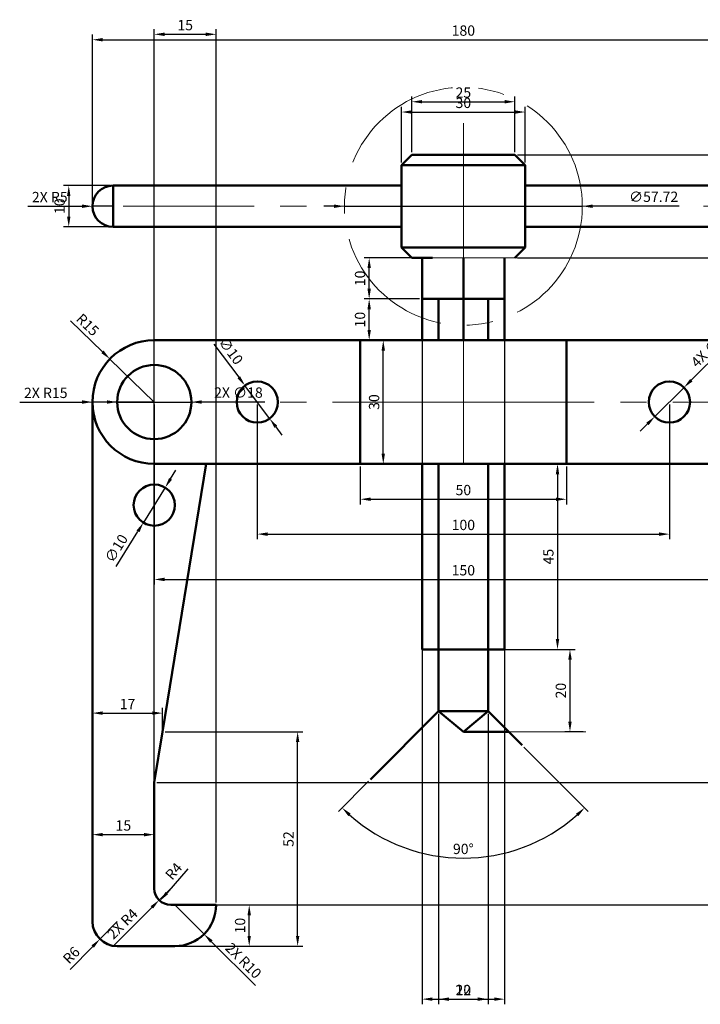
# Model space of a CAD drawing. Units: millimetres. Extents: x 5897 to 6166, y 4290 to 4529.
# Tile 1 of 2: x 5897 to 6062, y 4290 to 4529. Entities that reach past the tile are written whole.
import ezdxf

# ---------------------------------------------------------------- set-up
doc = ezdxf.new("R2010")
doc.units = ezdxf.units.MM
doc.linetypes.add('CENTER', pattern=[50.8, 31.75, -6.35, 6.35, -6.35])
for name, color, linetype, lineweight in [('M-CNTR', 1, 'CENTER', 18), ('M-CONS', 8, 'Continuous', 13), ('M-DIMS', 2, 'Continuous', 25), ('M-OUTL', 7, 'Continuous', 50)]:
    doc.layers.add(name, color=color, linetype=linetype, lineweight=lineweight)
doc.styles.get("Standard").update_dxf_attribs({"font": 'arial.ttf'})
doc.dimstyles.new('ISO-25', dxfattribs={"dimtxt": 2.5, "dimasz": 2.5, "dimexe": 1.25, "dimexo": 0.625, "dimtad": 1, "dimtxsty": 'Standard', "dimcen": 2.5, "dimadec": 0, "dimazin": 0, "dimtfac": 1, "dimtmove": 0, "dimatfit": 3, "dimfxl": 1, "dimarcsym": 0})

# ---------------------------------------------------------------- blocks, each defined once
blk = doc.blocks.new('*D1')
at = {"layer": 'Defpoints', "color": 0, "transparency": 16777216}
for p in [(5998.69, 4361.5), (6010.69, 4361.5), (6018.96, 4353.23), (5982.15, 4344.96), (5993.91, 4327.29)]:
    blk.add_point(p, dxfattribs=at)
at = {"layer": 'M-DIMS', "color": 0, "lineweight": -2, "transparency": 16777216}
for p, q in [((6019.4, 4352.79), (6035.01, 4337.18)), ((5981.7, 4344.52), (5974.37, 4337.18))]:
    blk.add_line(p, q, dxfattribs=at)
blk.add_arc((6004.69, 4367.5), 41.63, 228.4413, 311.5587, dxfattribs=at)
at = {"layer": 'M-DIMS', "color": 0, "transparency": 16777216}
for points in [[(5976.79, 4336.05), (5977.36, 4336.65), (5975.25, 4338.07)], [(6032.02, 4336.65), (6032.59, 4336.05), (6034.12, 4338.07)]]:
    blk.add_solid(points, dxfattribs=at)
at = {"layer": 'M-DIMS', "color": 0, "transparency": 16777216, "insert": (6004.69, 4327.77), "char_height": 2.5, "attachment_point": 5}
blk.add_mtext('90°', dxfattribs=at)
blk = doc.blocks.new('*D2')
at = {"layer": 'Defpoints', "color": 0, "transparency": 16777216}
for p in [(6010.69, 4376.5), (6030.56, 4356.5), (6034.41, 4356.5)]:
    blk.add_point(p, dxfattribs=at)
at = {"layer": 'M-DIMS', "color": 0, "lineweight": -2, "transparency": 16777216}
for p, q in [((6011.31, 4376.5), (6031.81, 4376.5)), ((6030.56, 4374), (6030.56, 4359)), ((6033.78, 4356.5), (6029.31, 4356.5))]:
    blk.add_line(p, q, dxfattribs=at)
at = {"layer": 'M-DIMS', "color": 0, "transparency": 16777216}
for points in [[(6030.15, 4374), (6030.98, 4374), (6030.56, 4376.5)], [(6030.15, 4359), (6030.98, 4359), (6030.56, 4356.5)]]:
    blk.add_solid(points, dxfattribs=at)
at = {"layer": 'M-DIMS', "color": 0, "transparency": 16777216, "insert": (6028.66, 4366.5), "char_height": 2.5, "attachment_point": 5, "rotation": 90}
blk.add_mtext('20', dxfattribs=at)
blk = doc.blocks.new('*D3')
at = {"layer": 'Defpoints', "color": 0, "transparency": 16777216}
for p in [(5931.69, 4356.5), (5964.48, 4356.5), (5927.69, 4304.5)]:
    blk.add_point(p, dxfattribs=at)
at = {"layer": 'M-DIMS', "color": 0, "lineweight": -2, "transparency": 16777216}
for p, q in [((5932.31, 4356.5), (5965.73, 4356.5)), ((5964.48, 4307), (5964.48, 4354)), ((5928.31, 4304.5), (5965.73, 4304.5))]:
    blk.add_line(p, q, dxfattribs=at)
at = {"layer": 'M-DIMS', "color": 0, "transparency": 16777216}
for points in [[(5964.06, 4354), (5964.89, 4354), (5964.48, 4356.5)], [(5964.06, 4307), (5964.89, 4307), (5964.48, 4304.5)]]:
    blk.add_solid(points, dxfattribs=at)
at = {"layer": 'M-DIMS', "color": 0, "transparency": 16777216, "insert": (5962.58, 4330.5), "char_height": 2.5, "attachment_point": 5, "rotation": 90}
blk.add_mtext('52', dxfattribs=at)
blk = doc.blocks.new('*D4')
at = {"layer": 'Defpoints', "color": 0, "transparency": 16777216}
for p in [(5933.69, 4314.5), (5952.73, 4314.5), (5927.69, 4304.5)]:
    blk.add_point(p, dxfattribs=at)
at = {"layer": 'M-DIMS', "color": 0, "lineweight": -2, "transparency": 16777216}
for p, q in [((5934.31, 4314.5), (5953.98, 4314.5)), ((5952.73, 4307), (5952.73, 4312)), ((5928.31, 4304.5), (5953.98, 4304.5))]:
    blk.add_line(p, q, dxfattribs=at)
at = {"layer": 'M-DIMS', "color": 0, "transparency": 16777216}
for points in [[(5952.31, 4312), (5953.14, 4312), (5952.73, 4314.5)], [(5952.31, 4307), (5953.14, 4307), (5952.73, 4304.5)]]:
    blk.add_solid(points, dxfattribs=at)
at = {"layer": 'M-DIMS', "color": 0, "transparency": 16777216, "insert": (5950.83, 4309.5), "char_height": 2.5, "attachment_point": 5, "rotation": 90}
blk.add_mtext('10', dxfattribs=at)
blk = doc.blocks.new('*D5')
at = {"layer": 'Defpoints', "color": 0, "transparency": 16777216}
for p in [(5914.69, 4341.08), (5929.69, 4341.08), (5929.69, 4331.56)]:
    blk.add_point(p, dxfattribs=at)
at = {"layer": 'M-DIMS', "color": 0, "lineweight": -2, "transparency": 16777216}
for p, q in [((5914.69, 4340.45), (5914.69, 4330.31)), ((5929.69, 4340.45), (5929.69, 4330.31)), ((5917.19, 4331.56), (5927.19, 4331.56))]:
    blk.add_line(p, q, dxfattribs=at)
at = {"layer": 'M-DIMS', "color": 0, "transparency": 16777216}
for points in [[(5917.19, 4331.97), (5917.19, 4331.14), (5914.69, 4331.56)], [(5927.19, 4331.97), (5927.19, 4331.14), (5929.69, 4331.56)]]:
    blk.add_solid(points, dxfattribs=at)
at = {"layer": 'M-DIMS', "color": 0, "transparency": 16777216, "insert": (5922.19, 4333.46), "char_height": 2.5, "attachment_point": 5}
blk.add_mtext('15', dxfattribs=at)
blk = doc.blocks.new('*D6')
at = {"layer": 'Defpoints', "color": 0, "transparency": 16777216}
for p in [(5931.69, 4361.04), (5914.69, 4356.5), (5931.69, 4356.5)]:
    blk.add_point(p, dxfattribs=at)
at = {"layer": 'M-DIMS', "color": 0, "lineweight": -2, "transparency": 16777216}
for p, q in [((5914.69, 4357.13), (5914.69, 4362.29)), ((5931.69, 4357.13), (5931.69, 4362.29)), ((5917.19, 4361.04), (5929.19, 4361.04))]:
    blk.add_line(p, q, dxfattribs=at)
at = {"layer": 'M-DIMS', "color": 0, "transparency": 16777216}
for points in [[(5917.19, 4361.46), (5917.19, 4360.62), (5914.69, 4361.04)], [(5929.19, 4361.46), (5929.19, 4360.62), (5931.69, 4361.04)]]:
    blk.add_solid(points, dxfattribs=at)
at = {"layer": 'M-DIMS', "color": 0, "transparency": 16777216, "insert": (5923.19, 4362.92), "char_height": 2.5, "attachment_point": 5}
blk.add_mtext('17', dxfattribs=at)
blk = doc.blocks.new('*D7')
at = {"layer": 'Defpoints', "color": 0, "transparency": 16777216}
for p in [(5979.69, 4421.5), (6029.69, 4421.5), (6029.69, 4412.92)]:
    blk.add_point(p, dxfattribs=at)
at = {"layer": 'M-DIMS', "color": 0, "lineweight": -2, "transparency": 16777216}
for p, q in [((5979.69, 4420.88), (5979.69, 4411.67)), ((6029.69, 4420.88), (6029.69, 4411.67)), ((5982.19, 4412.92), (6027.19, 4412.92))]:
    blk.add_line(p, q, dxfattribs=at)
at = {"layer": 'M-DIMS', "color": 0, "transparency": 16777216}
for points in [[(5982.19, 4413.34), (5982.19, 4412.51), (5979.69, 4412.92)], [(6027.19, 4413.34), (6027.19, 4412.51), (6029.69, 4412.92)]]:
    blk.add_solid(points, dxfattribs=at)
at = {"layer": 'M-DIMS', "color": 0, "transparency": 16777216, "insert": (6004.69, 4414.83), "char_height": 2.5, "attachment_point": 5}
blk.add_mtext('50', dxfattribs=at)
blk = doc.blocks.new('*D8')
at = {"layer": 'Defpoints', "color": 0, "transparency": 16777216}
for p in [(5954.69, 4436.5), (6054.69, 4436.5), (6054.69, 4404.46)]:
    blk.add_point(p, dxfattribs=at)
at = {"layer": 'M-DIMS', "color": 0, "lineweight": -2, "transparency": 16777216}
for p, q in [((5954.69, 4435.88), (5954.69, 4403.21)), ((6054.69, 4435.88), (6054.69, 4403.21)), ((5957.19, 4404.46), (6052.19, 4404.46))]:
    blk.add_line(p, q, dxfattribs=at)
at = {"layer": 'M-DIMS', "color": 0, "transparency": 16777216}
for points in [[(5957.19, 4404.88), (5957.19, 4404.04), (5954.69, 4404.46)], [(6052.19, 4404.88), (6052.19, 4404.04), (6054.69, 4404.46)]]:
    blk.add_solid(points, dxfattribs=at)
at = {"layer": 'M-DIMS', "color": 0, "transparency": 16777216, "insert": (6004.69, 4406.36), "char_height": 2.5, "attachment_point": 5}
blk.add_mtext('100', dxfattribs=at)
blk = doc.blocks.new('*D9')
at = {"layer": 'Defpoints', "color": 0, "transparency": 16777216}
for p in [(5929.69, 4436.5), (6079.69, 4436.5), (6079.69, 4393.47)]:
    blk.add_point(p, dxfattribs=at)
at = {"layer": 'M-DIMS', "color": 0, "lineweight": -2, "transparency": 16777216}
for p, q in [((5929.69, 4435.88), (5929.69, 4392.22)), ((6079.69, 4435.88), (6079.69, 4392.22)), ((5932.19, 4393.47), (6077.19, 4393.47))]:
    blk.add_line(p, q, dxfattribs=at)
at = {"layer": 'M-DIMS', "color": 0, "transparency": 16777216}
for points in [[(5932.19, 4393.89), (5932.19, 4393.06), (5929.69, 4393.47)], [(6077.19, 4393.89), (6077.19, 4393.06), (6079.69, 4393.47)]]:
    blk.add_solid(points, dxfattribs=at)
at = {"layer": 'M-DIMS', "color": 0, "transparency": 16777216, "insert": (6004.69, 4395.37), "char_height": 2.5, "attachment_point": 5}
blk.add_mtext('150', dxfattribs=at)
blk = doc.blocks.new('*D10')
at = {"layer": 'Defpoints', "color": 0, "transparency": 16777216}
for p in [(6094.69, 4524.39), (5914.69, 4484), (6094.69, 4484)]:
    blk.add_point(p, dxfattribs=at)
at = {"layer": 'M-DIMS', "color": 0, "lineweight": -2, "transparency": 16777216}
for p, q in [((5914.69, 4484.63), (5914.69, 4525.64)), ((5917.19, 4524.39), (6092.19, 4524.39)), ((6094.69, 4484.63), (6094.69, 4525.64))]:
    blk.add_line(p, q, dxfattribs=at)
at = {"layer": 'M-DIMS', "color": 0, "transparency": 16777216}
for points in [[(5917.19, 4524.81), (5917.19, 4523.97), (5914.69, 4524.39)], [(6092.19, 4524.81), (6092.19, 4523.97), (6094.69, 4524.39)]]:
    blk.add_solid(points, dxfattribs=at)
at = {"layer": 'M-DIMS', "color": 0, "transparency": 16777216, "insert": (6004.69, 4526.29), "char_height": 2.5, "attachment_point": 5}
blk.add_mtext('180', dxfattribs=at)
blk = doc.blocks.new('*D11')
at = {"layer": 'Defpoints', "color": 0, "transparency": 16777216}
for p in [(5919.69, 4489), (5908.94, 4479), (5919.69, 4479)]:
    blk.add_point(p, dxfattribs=at)
at = {"layer": 'M-DIMS', "color": 0, "lineweight": -2, "transparency": 16777216}
for p, q in [((5919.06, 4489), (5907.69, 4489)), ((5908.94, 4486.5), (5908.94, 4481.5)), ((5919.06, 4479), (5907.69, 4479))]:
    blk.add_line(p, q, dxfattribs=at)
at = {"layer": 'M-DIMS', "color": 0, "transparency": 16777216}
for points in [[(5908.52, 4486.5), (5909.35, 4486.5), (5908.94, 4489)], [(5908.52, 4481.5), (5909.35, 4481.5), (5908.94, 4479)]]:
    blk.add_solid(points, dxfattribs=at)
at = {"layer": 'M-DIMS', "color": 0, "transparency": 16777216, "insert": (5907.04, 4484), "char_height": 2.5, "attachment_point": 5, "rotation": 90}
blk.add_mtext('10', dxfattribs=at)
blk = doc.blocks.new('*D12')
at = {"layer": 'Defpoints', "color": 0, "transparency": 16777216}
for p in [(5920.69, 4310.5), (5916.49, 4306.21)]:
    blk.add_point(p, dxfattribs=at)
at = {"layer": 'M-DIMS', "color": 0, "lineweight": -2, "transparency": 16777216}
for p, q in [((5920.69, 4310.5), (5916.49, 4306.21)), ((5909.31, 4298.86), (5914.75, 4304.42))]:
    blk.add_line(p, q, dxfattribs=at)
at = {"layer": 'M-DIMS', "color": 0, "transparency": 16777216}
blk.add_solid([(5914.45, 4304.71), (5915.04, 4304.13), (5916.49, 4306.21)], dxfattribs=at)
at = {"layer": 'M-DIMS', "color": 0, "transparency": 16777216, "insert": (5909.79, 4302.08), "char_height": 2.5, "attachment_point": 5, "rotation": 45.6503}
blk.add_mtext('R6', dxfattribs=at)
blk = doc.blocks.new('*D13')
at = {"layer": 'Defpoints', "color": 0, "transparency": 16777216}
for p in [(5933.69, 4318.5), (5931.07, 4315.48)]:
    blk.add_point(p, dxfattribs=at)
at = {"layer": 'M-DIMS', "color": 0, "lineweight": -2, "transparency": 16777216}
blk.add_line((5937.8, 4323.24), (5932.71, 4317.37), dxfattribs=at)
at = {"layer": 'M-DIMS', "color": 0, "transparency": 16777216}
blk.add_solid([(5932.39, 4317.64), (5933.02, 4317.1), (5931.07, 4315.48)], dxfattribs=at)
at = {"layer": 'M-DIMS', "color": 0, "transparency": 16777216, "insert": (5934.65, 4322.48), "char_height": 2.5, "attachment_point": 5, "rotation": 49.0832}
blk.add_mtext('R4', dxfattribs=at)
blk = doc.blocks.new('*D16')
at = {"layer": 'Defpoints', "color": 0, "transparency": 16777216}
for p in [(5951.69, 4440.51), (5957.68, 4432.5)]:
    blk.add_point(p, dxfattribs=at)
at = {"layer": 'M-DIMS', "color": 0, "lineweight": -2, "transparency": 16777216}
for p, q in [((5944.18, 4450.55), (5950.19, 4442.51)), ((5957.68, 4432.5), (5951.69, 4440.51)), ((5959.18, 4430.5), (5960.68, 4428.49))]:
    blk.add_line(p, q, dxfattribs=at)
at = {"layer": 'M-DIMS', "color": 0, "transparency": 16777216}
for points in [[(5950.53, 4442.76), (5949.86, 4442.26), (5951.69, 4440.51)], [(5959.51, 4430.75), (5958.85, 4430.25), (5957.68, 4432.5)]]:
    blk.add_solid(points, dxfattribs=at)
at = {"layer": 'M-DIMS', "color": 0, "transparency": 16777216, "insert": (5948.02, 4448.71), "char_height": 2.5, "attachment_point": 5, "rotation": 306.8024}
blk.add_mtext('∅10', dxfattribs=at)
blk = doc.blocks.new('*D17')
at = {"layer": 'Defpoints', "color": 0, "transparency": 16777216}
for p in [(5932.32, 4415.75), (5927.05, 4407.25)]:
    blk.add_point(p, dxfattribs=at)
at = {"layer": 'M-DIMS', "color": 0, "lineweight": -2, "transparency": 16777216}
for p, q in [((5933.64, 4417.87), (5934.96, 4420)), ((5932.32, 4415.75), (5927.05, 4407.25)), ((5920.44, 4396.6), (5925.73, 4405.13))]:
    blk.add_line(p, q, dxfattribs=at)
at = {"layer": 'M-DIMS', "color": 0, "transparency": 16777216}
for points in [[(5933.29, 4418.09), (5934, 4417.65), (5932.32, 4415.75)], [(5925.38, 4405.35), (5926.09, 4404.91), (5927.05, 4407.25)]]:
    blk.add_solid(points, dxfattribs=at)
at = {"layer": 'M-DIMS', "color": 0, "transparency": 16777216, "insert": (5920.75, 4400.84), "char_height": 2.5, "attachment_point": 5, "rotation": 58.1703}
blk.add_mtext('∅10', dxfattribs=at)
blk = doc.blocks.new('*D18')
at = {"layer": 'Defpoints', "color": 0, "transparency": 16777216}
for p in [(5979.69, 4451.5), (5985.26, 4451.5), (5979.69, 4421.5)]:
    blk.add_point(p, dxfattribs=at)
at = {"layer": 'M-DIMS', "color": 0, "lineweight": -2, "transparency": 16777216}
for p, q in [((5980.31, 4451.5), (5986.51, 4451.5)), ((5985.26, 4424), (5985.26, 4449)), ((5980.31, 4421.5), (5986.51, 4421.5))]:
    blk.add_line(p, q, dxfattribs=at)
at = {"layer": 'M-DIMS', "color": 0, "transparency": 16777216}
for points in [[(5984.84, 4449), (5985.67, 4449), (5985.26, 4451.5)], [(5984.84, 4424), (5985.67, 4424), (5985.26, 4421.5)]]:
    blk.add_solid(points, dxfattribs=at)
at = {"layer": 'M-DIMS', "color": 0, "transparency": 16777216, "insert": (5983.35, 4436.5), "char_height": 2.5, "attachment_point": 5, "rotation": 90}
blk.add_mtext('30', dxfattribs=at)
blk = doc.blocks.new('*D19')
at = {"layer": 'Defpoints', "color": 0, "transparency": 16777216}
for p in [(5918.91, 4446.94), (5929.69, 4436.5)]:
    blk.add_point(p, dxfattribs=at)
at = {"layer": 'M-DIMS', "color": 0, "lineweight": -2, "transparency": 16777216}
for p, q in [((5909.38, 4456.18), (5917.12, 4448.68)), ((5929.69, 4436.5), (5918.91, 4446.94))]:
    blk.add_line(p, q, dxfattribs=at)
at = {"layer": 'M-DIMS', "color": 0, "transparency": 16777216}
blk.add_solid([(5917.41, 4448.98), (5916.83, 4448.38), (5918.91, 4446.94)], dxfattribs=at)
at = {"layer": 'M-DIMS', "color": 0, "transparency": 16777216, "insert": (5913.3, 4455.02), "char_height": 2.5, "attachment_point": 5, "rotation": 315.9139}
blk.add_mtext('R15', dxfattribs=at)
blk = doc.blocks.new('*D20')
at = {"layer": 'Defpoints', "color": 0, "transparency": 16777216}
for p in [(6017.19, 4496.5), (6118.15, 4496.5), (6094.69, 4484)]:
    blk.add_point(p, dxfattribs=at)
at = {"layer": 'M-DIMS', "color": 0, "lineweight": -2, "transparency": 16777216}
for p, q in [((6017.81, 4496.5), (6119.4, 4496.5)), ((6118.15, 4486.5), (6118.15, 4494)), ((6095.31, 4484), (6119.4, 4484))]:
    blk.add_line(p, q, dxfattribs=at)
at = {"layer": 'M-DIMS', "color": 0, "transparency": 16777216}
for points in [[(6117.73, 4494), (6118.57, 4494), (6118.15, 4496.5)], [(6117.73, 4486.5), (6118.57, 4486.5), (6118.15, 4484)]]:
    blk.add_solid(points, dxfattribs=at)
at = {"layer": 'M-DIMS', "color": 0, "transparency": 16777216, "insert": (6116.25, 4490.25), "char_height": 2.5, "attachment_point": 5, "rotation": 90}
blk.add_mtext('12.5', dxfattribs=at)
blk = doc.blocks.new('*D21')
at = {"layer": 'Defpoints', "color": 0, "transparency": 16777216}
for p in [(6094.69, 4484), (6118.15, 4484), (6017.19, 4471.5)]:
    blk.add_point(p, dxfattribs=at)
at = {"layer": 'M-DIMS', "color": 0, "lineweight": -2, "transparency": 16777216}
for p, q in [((6095.31, 4484), (6119.4, 4484)), ((6118.15, 4474), (6118.15, 4481.5)), ((6017.81, 4471.5), (6119.4, 4471.5))]:
    blk.add_line(p, q, dxfattribs=at)
at = {"layer": 'M-DIMS', "color": 0, "transparency": 16777216}
for points in [[(6117.73, 4481.5), (6118.57, 4481.5), (6118.15, 4484)], [(6117.73, 4474), (6118.57, 4474), (6118.15, 4471.5)]]:
    blk.add_solid(points, dxfattribs=at)
at = {"layer": 'M-DIMS', "color": 0, "transparency": 16777216, "insert": (6116.25, 4477.75), "char_height": 2.5, "attachment_point": 5, "rotation": 90}
blk.add_mtext('12.5', dxfattribs=at)
blk = doc.blocks.new('*D22')
at = {"layer": 'Defpoints', "color": 0, "transparency": 16777216}
for p in [(6014.69, 4421.5), (6014.69, 4376.5), (6027.54, 4376.5)]:
    blk.add_point(p, dxfattribs=at)
at = {"layer": 'M-DIMS', "color": 0, "lineweight": -2, "transparency": 16777216}
for p, q in [((6015.31, 4421.5), (6028.79, 4421.5)), ((6027.54, 4419), (6027.54, 4379)), ((6015.31, 4376.5), (6028.79, 4376.5))]:
    blk.add_line(p, q, dxfattribs=at)
at = {"layer": 'M-DIMS', "color": 0, "transparency": 16777216}
for points in [[(6027.12, 4419), (6027.95, 4419), (6027.54, 4421.5)], [(6027.12, 4379), (6027.95, 4379), (6027.54, 4376.5)]]:
    blk.add_solid(points, dxfattribs=at)
at = {"layer": 'M-DIMS', "color": 0, "transparency": 16777216, "insert": (6025.64, 4399), "char_height": 2.5, "attachment_point": 5, "rotation": 90}
blk.add_mtext('45', dxfattribs=at)
blk = doc.blocks.new('*D23')
at = {"layer": 'Defpoints', "color": 0, "transparency": 16777216}
for p in [(5981.84, 4461.5), (5994.69, 4461.5), (5994.69, 4451.5)]:
    blk.add_point(p, dxfattribs=at)
at = {"layer": 'M-DIMS', "color": 0, "lineweight": -2, "transparency": 16777216}
for p, q in [((5994.06, 4461.5), (5980.59, 4461.5)), ((5981.84, 4454), (5981.84, 4459)), ((5994.06, 4451.5), (5980.59, 4451.5))]:
    blk.add_line(p, q, dxfattribs=at)
at = {"layer": 'M-DIMS', "color": 0, "transparency": 16777216}
for points in [[(5981.42, 4459), (5982.25, 4459), (5981.84, 4461.5)], [(5981.42, 4454), (5982.25, 4454), (5981.84, 4451.5)]]:
    blk.add_solid(points, dxfattribs=at)
at = {"layer": 'M-DIMS', "color": 0, "transparency": 16777216, "insert": (5979.94, 4456.5), "char_height": 2.5, "attachment_point": 5, "rotation": 90}
blk.add_mtext('10', dxfattribs=at)
blk = doc.blocks.new('*D24')
at = {"layer": 'Defpoints', "color": 0, "transparency": 16777216}
for p in [(5981.84, 4471.5), (5994.69, 4471.5), (5994.69, 4461.5)]:
    blk.add_point(p, dxfattribs=at)
at = {"layer": 'M-DIMS', "color": 0, "lineweight": -2, "transparency": 16777216}
for p, q in [((5994.06, 4471.5), (5980.59, 4471.5)), ((5981.84, 4464), (5981.84, 4469)), ((5994.06, 4461.5), (5980.59, 4461.5))]:
    blk.add_line(p, q, dxfattribs=at)
at = {"layer": 'M-DIMS', "color": 0, "transparency": 16777216}
for points in [[(5981.42, 4469), (5982.25, 4469), (5981.84, 4471.5)], [(5981.42, 4464), (5982.25, 4464), (5981.84, 4461.5)]]:
    blk.add_solid(points, dxfattribs=at)
at = {"layer": 'M-DIMS', "color": 0, "transparency": 16777216, "insert": (5979.94, 4466.5), "char_height": 2.5, "attachment_point": 5, "rotation": 90}
blk.add_mtext('10', dxfattribs=at)
blk = doc.blocks.new('*D25')
at = {"layer": 'Defpoints', "color": 0, "transparency": 16777216}
for p in [(5929.69, 4344.19), (5944.69, 4314.5), (6118.15, 4314.5)]:
    blk.add_point(p, dxfattribs=at)
at = {"layer": 'M-DIMS', "color": 0, "lineweight": -2, "transparency": 16777216}
for p, q in [((5930.31, 4344.19), (6119.4, 4344.19)), ((6118.15, 4341.69), (6118.15, 4317)), ((5945.31, 4314.5), (6119.4, 4314.5))]:
    blk.add_line(p, q, dxfattribs=at)
at = {"layer": 'M-DIMS', "color": 0, "transparency": 16777216}
for points in [[(6117.73, 4341.69), (6118.57, 4341.69), (6118.15, 4344.19)], [(6117.73, 4317), (6118.57, 4317), (6118.15, 4314.5)]]:
    blk.add_solid(points, dxfattribs=at)
at = {"layer": 'M-DIMS', "color": 0, "transparency": 16777216, "insert": (6116.25, 4329.35), "char_height": 2.5, "attachment_point": 5, "rotation": 90}
blk.add_mtext('29.69', dxfattribs=at)
blk = doc.blocks.new('*D26')
at = {"layer": 'Defpoints', "color": 0, "transparency": 16777216}
for p in [(5944.69, 4525.71), (5929.69, 4318.5), (5944.69, 4314.5)]:
    blk.add_point(p, dxfattribs=at)
at = {"layer": 'M-DIMS', "color": 0, "lineweight": -2, "transparency": 16777216}
for p, q in [((5929.69, 4319.13), (5929.69, 4526.96)), ((5944.69, 4315.13), (5944.69, 4526.96)), ((5932.19, 4525.71), (5942.19, 4525.71))]:
    blk.add_line(p, q, dxfattribs=at)
at = {"layer": 'M-DIMS', "color": 0, "transparency": 16777216}
for points in [[(5932.19, 4526.13), (5932.19, 4525.29), (5929.69, 4525.71)], [(5942.19, 4526.13), (5942.19, 4525.29), (5944.69, 4525.71)]]:
    blk.add_solid(points, dxfattribs=at)
at = {"layer": 'M-DIMS', "color": 0, "transparency": 16777216, "insert": (5937.19, 4527.61), "char_height": 2.5, "attachment_point": 5}
blk.add_mtext('15', dxfattribs=at)
blk = doc.blocks.new('*D27')
at = {"layer": 'Defpoints', "color": 0, "transparency": 16777216}
for p in [(6019.69, 4506.85), (5989.69, 4494), (6019.69, 4494)]:
    blk.add_point(p, dxfattribs=at)
at = {"layer": 'M-DIMS', "color": 0, "lineweight": -2, "transparency": 16777216}
for p, q in [((5989.69, 4494.63), (5989.69, 4508.1)), ((6019.69, 4494.63), (6019.69, 4508.1)), ((5992.19, 4506.85), (6017.19, 4506.85))]:
    blk.add_line(p, q, dxfattribs=at)
at = {"layer": 'M-DIMS', "color": 0, "transparency": 16777216}
for points in [[(5992.19, 4507.27), (5992.19, 4506.44), (5989.69, 4506.85)], [(6017.19, 4507.27), (6017.19, 4506.44), (6019.69, 4506.85)]]:
    blk.add_solid(points, dxfattribs=at)
at = {"layer": 'M-DIMS', "color": 0, "transparency": 16777216, "insert": (6004.69, 4508.75), "char_height": 2.5, "attachment_point": 5}
blk.add_mtext('30', dxfattribs=at)
blk = doc.blocks.new('*D28')
at = {"layer": 'Defpoints', "color": 0, "transparency": 16777216}
for p in [(6017.19, 4509.35), (5992.19, 4496.5), (6017.19, 4496.5)]:
    blk.add_point(p, dxfattribs=at)
at = {"layer": 'M-DIMS', "color": 0, "lineweight": -2, "transparency": 16777216}
for p, q in [((5992.19, 4497.13), (5992.19, 4510.6)), ((6017.19, 4497.13), (6017.19, 4510.6)), ((5994.69, 4509.35), (6014.69, 4509.35))]:
    blk.add_line(p, q, dxfattribs=at)
at = {"layer": 'M-DIMS', "color": 0, "transparency": 16777216}
for points in [[(5994.69, 4509.77), (5994.69, 4508.94), (5992.19, 4509.35)], [(6014.69, 4509.77), (6014.69, 4508.94), (6017.19, 4509.35)]]:
    blk.add_solid(points, dxfattribs=at)
at = {"layer": 'M-DIMS', "color": 0, "transparency": 16777216, "insert": (6004.69, 4511.25), "char_height": 2.5, "attachment_point": 5}
blk.add_mtext('25', dxfattribs=at)
blk = doc.blocks.new('*D29')
at = {"layer": 'Defpoints', "color": 0, "transparency": 16777216}
for p in [(5994.69, 4471.5), (6014.69, 4471.5), (6014.69, 4291.65)]:
    blk.add_point(p, dxfattribs=at)
at = {"layer": 'M-DIMS', "color": 0, "lineweight": -2, "transparency": 16777216}
for p, q in [((5994.69, 4470.88), (5994.69, 4290.4)), ((6014.69, 4470.88), (6014.69, 4290.4)), ((5997.19, 4291.65), (6012.19, 4291.65))]:
    blk.add_line(p, q, dxfattribs=at)
at = {"layer": 'M-DIMS', "color": 0, "transparency": 16777216}
for points in [[(5997.19, 4292.07), (5997.19, 4291.24), (5994.69, 4291.65)], [(6012.19, 4292.07), (6012.19, 4291.24), (6014.69, 4291.65)]]:
    blk.add_solid(points, dxfattribs=at)
at = {"layer": 'M-DIMS', "color": 0, "transparency": 16777216, "insert": (6004.69, 4293.55), "char_height": 2.5, "attachment_point": 5}
blk.add_mtext('20', dxfattribs=at)
blk = doc.blocks.new('*D30')
at = {"layer": 'Defpoints', "color": 0, "transparency": 16777216}
for p in [(5998.69, 4361.5), (6010.69, 4361.5), (6010.69, 4291.65)]:
    blk.add_point(p, dxfattribs=at)
at = {"layer": 'M-DIMS', "color": 0, "lineweight": -2, "transparency": 16777216}
for p, q in [((5998.69, 4360.88), (5998.69, 4290.4)), ((6010.69, 4360.88), (6010.69, 4290.4)), ((6001.19, 4291.65), (6008.19, 4291.65))]:
    blk.add_line(p, q, dxfattribs=at)
at = {"layer": 'M-DIMS', "color": 0, "transparency": 16777216}
for points in [[(6001.19, 4292.07), (6001.19, 4291.24), (5998.69, 4291.65)], [(6008.19, 4292.07), (6008.19, 4291.24), (6010.69, 4291.65)]]:
    blk.add_solid(points, dxfattribs=at)
at = {"layer": 'M-DIMS', "color": 0, "transparency": 16777216, "insert": (6004.69, 4293.53), "char_height": 2.5, "attachment_point": 5}
blk.add_mtext('12', dxfattribs=at)
blk = doc.blocks.new('*D31')
at = {"layer": 'Defpoints', "color": 0, "transparency": 16777216}
for p in [(5975.83, 4484), (6033.55, 4484)]:
    blk.add_point(p, dxfattribs=at)
at = {"layer": 'M-DIMS', "color": 0, "lineweight": -2, "transparency": 16777216}
for p, q in [((5973.33, 4484), (5970.83, 4484)), ((5975.83, 4484), (6033.55, 4484)), ((6057.05, 4484), (6036.05, 4484))]:
    blk.add_line(p, q, dxfattribs=at)
at = {"layer": 'M-DIMS', "color": 0, "transparency": 16777216}
for points in [[(5973.33, 4484.42), (5973.33, 4483.59), (5975.83, 4484)], [(6036.05, 4484.42), (6036.05, 4483.59), (6033.55, 4484)]]:
    blk.add_solid(points, dxfattribs=at)
at = {"layer": 'M-DIMS', "color": 0, "transparency": 16777216, "insert": (6050.86, 4485.97), "char_height": 2.5, "attachment_point": 5, "rotation": 0.0001}
blk.add_mtext('∅57.72', dxfattribs=at)
blk = doc.blocks.new('*D32')
at = {"layer": 'Defpoints', "color": 0, "transparency": 16777216}
for p in [(5914.69, 4436.5), (5929.69, 4436.5)]:
    blk.add_point(p, dxfattribs=at)
at = {"layer": 'M-DIMS', "color": 0, "lineweight": -2, "transparency": 16777216}
for p, q in [((5897.03, 4436.5), (5912.19, 4436.5)), ((5929.69, 4436.5), (5914.69, 4436.5))]:
    blk.add_line(p, q, dxfattribs=at)
at = {"layer": 'M-DIMS', "color": 0, "transparency": 16777216}
blk.add_solid([(5912.19, 4436.92), (5912.19, 4436.09), (5914.69, 4436.5)], dxfattribs=at)
at = {"layer": 'M-DIMS', "color": 0, "transparency": 16777216, "insert": (5903.36, 4438.4), "char_height": 2.5, "attachment_point": 5, "rotation": 359.9998}
blk.add_mtext('2X R15', dxfattribs=at)
blk = doc.blocks.new('*D33')
at = {"layer": 'Defpoints', "color": 0, "transparency": 16777216}
for p in [(5934.69, 4314.5), (5941.76, 4307.43)]:
    blk.add_point(p, dxfattribs=at)
at = {"layer": 'M-DIMS', "color": 0, "lineweight": -2, "transparency": 16777216}
for p, q in [((5934.69, 4314.5), (5941.76, 4307.43)), ((5954.23, 4294.97), (5943.53, 4305.66))]:
    blk.add_line(p, q, dxfattribs=at)
at = {"layer": 'M-DIMS', "color": 0, "transparency": 16777216}
blk.add_solid([(5943.82, 4305.96), (5943.23, 4305.37), (5941.76, 4307.43)], dxfattribs=at)
at = {"layer": 'M-DIMS', "color": 0, "transparency": 16777216, "insert": (5951.1, 4300.78), "char_height": 2.5, "attachment_point": 5, "rotation": 315.0015}
blk.add_mtext('2X R10', dxfattribs=at)
blk = doc.blocks.new('*D34')
at = {"layer": 'Defpoints', "color": 0, "transparency": 16777216}
for p in [(5920.69, 4436.5), (5938.69, 4436.5)]:
    blk.add_point(p, dxfattribs=at)
at = {"layer": 'M-DIMS', "color": 0, "lineweight": -2, "transparency": 16777216}
for p, q in [((5918.19, 4436.5), (5915.69, 4436.5)), ((5920.69, 4436.5), (5938.69, 4436.5)), ((5956.53, 4436.5), (5941.19, 4436.5))]:
    blk.add_line(p, q, dxfattribs=at)
at = {"layer": 'M-DIMS', "color": 0, "transparency": 16777216}
for points in [[(5918.19, 4436.92), (5918.19, 4436.09), (5920.69, 4436.5)], [(5941.19, 4436.92), (5941.19, 4436.09), (5938.69, 4436.5)]]:
    blk.add_solid(points, dxfattribs=at)
at = {"layer": 'M-DIMS', "color": 0, "transparency": 16777216, "insert": (5950.11, 4438.47), "char_height": 2.5, "attachment_point": 5, "rotation": 0.0003}
blk.add_mtext('2X ∅18', dxfattribs=at)
blk = doc.blocks.new('*D36')
at = {"layer": 'Defpoints', "color": 0, "transparency": 16777216}
for p in [(6058.23, 4440.03), (6051.14, 4432.97)]:
    blk.add_point(p, dxfattribs=at)
at = {"layer": 'M-DIMS', "color": 0, "lineweight": -2, "transparency": 16777216}
for p, q in [((6070.9, 4452.65), (6060, 4441.79)), ((6051.14, 4432.97), (6058.23, 4440.03)), ((6049.37, 4431.21), (6047.6, 4429.45))]:
    blk.add_line(p, q, dxfattribs=at)
at = {"layer": 'M-DIMS', "color": 0, "transparency": 16777216}
for points in [[(6059.71, 4442.09), (6060.3, 4441.5), (6058.23, 4440.03)], [(6049.08, 4431.5), (6049.67, 4430.91), (6051.14, 4432.97)]]:
    blk.add_solid(points, dxfattribs=at)
at = {"layer": 'M-DIMS', "color": 0, "transparency": 16777216, "insert": (6064.95, 4449.5), "char_height": 2.5, "attachment_point": 5, "rotation": 44.8833}
blk.add_mtext('4X ∅10', dxfattribs=at)
blk = doc.blocks.new('*D37')
at = {"layer": 'Defpoints', "color": 0, "transparency": 16777216}
for p in [(5914.69, 4484), (5919.69, 4484)]:
    blk.add_point(p, dxfattribs=at)
at = {"layer": 'M-DIMS', "color": 0, "lineweight": -2, "transparency": 16777216}
for p, q in [((5898.97, 4484), (5912.19, 4484)), ((5919.69, 4484), (5914.69, 4484))]:
    blk.add_line(p, q, dxfattribs=at)
at = {"layer": 'M-DIMS', "color": 0, "transparency": 16777216}
blk.add_solid([(5912.19, 4484.42), (5912.19, 4483.59), (5914.69, 4484)], dxfattribs=at)
at = {"layer": 'M-DIMS', "color": 0, "transparency": 16777216, "insert": (5904.33, 4485.9), "char_height": 2.5, "attachment_point": 5, "rotation": 359.9995}
blk.add_mtext('2X R5', dxfattribs=at)
blk = doc.blocks.new('*D38')
at = {"layer": 'Defpoints', "color": 0, "transparency": 16777216}
for p in [(5933.69, 4318.5), (5930.86, 4315.67)]:
    blk.add_point(p, dxfattribs=at)
at = {"layer": 'M-DIMS', "color": 0, "lineweight": -2, "transparency": 16777216}
for p, q in [((5933.69, 4318.5), (5930.86, 4315.67)), ((5919.77, 4304.58), (5929.09, 4313.91))]:
    blk.add_line(p, q, dxfattribs=at)
at = {"layer": 'M-DIMS', "color": 0, "transparency": 16777216}
blk.add_solid([(5928.8, 4314.2), (5929.39, 4313.61), (5930.86, 4315.67)], dxfattribs=at)
at = {"layer": 'M-DIMS', "color": 0, "transparency": 16777216, "insert": (5922.21, 4309.69), "char_height": 2.5, "attachment_point": 5, "rotation": 44.9926}
blk.add_mtext('2X R4', dxfattribs=at)

msp = doc.modelspace()

# ---------------------------------------------------------------- linework, layer by layer
at = {"layer": 'M-CNTR'}
for p, q in [((6004.688, 4496.502), (6004.688, 4504.117)), ((6004.688, 4471.502), (6004.688, 4496.502)), ((6004.688, 4484.002), (5914.688, 4484.002)), ((6094.688, 4484.002), (6004.688, 4484.002)), ((6004.688, 4451.502), (6004.688, 4471.502)), ((6004.688, 4451.502), (6004.688, 4461.502)), ((6004.688, 4451.502), (6004.688, 4421.502)), ((6004.688, 4436.502), (5905.344, 4436.502)), ((6004.688, 4436.502), (6105.301, 4436.502))]:
    msp.add_line(p, q, dxfattribs=at)
msp.add_circle((6004.688, 4484.002), 28.86, dxfattribs=at)
at = {"layer": 'M-CONS'}
for p, q in [((6165.744, 4471.502), (5997.188, 4471.502)), ((6004.688, 4471.502), (6165.744, 4471.502)), ((6004.688, 4356.502), (6034.406, 4356.502))]:
    msp.add_line(p, q, dxfattribs=at)
at = {"layer": 'M-OUTL'}
for p, q in [((5989.688, 4494.002), (5992.188, 4496.502)), ((5997.188, 4496.502), (5992.188, 4496.502)), ((6012.188, 4496.502), (5997.188, 4496.502)), ((6004.688, 4496.502), (6012.188, 4496.502)), ((6012.188, 4496.502), (6017.188, 4496.502)), ((6019.688, 4494.002), (6017.188, 4496.502)), ((5994.688, 4494.002), (5989.688, 4494.002)), ((5989.688, 4494.002), (5989.688, 4474.002)), ((5994.688, 4494.002), (6014.688, 4494.002)), ((6014.688, 4494.002), (6019.688, 4494.002)), ((6019.688, 4494.002), (6019.688, 4474.002)), ((5919.688, 4489.002), (5989.688, 4489.002)), ((5919.688, 4484.002), (5919.688, 4489.002)), ((5919.688, 4489.002), (5919.688, 4479.002)), ((6019.688, 4489.002), (6089.688, 4489.002)), ((5989.688, 4479.002), (5919.688, 4479.002)), ((6089.688, 4479.002), (6019.688, 4479.002)), ((5994.688, 4474.002), (5989.688, 4474.002)), ((5989.688, 4474.002), (5992.188, 4471.502)), ((6014.688, 4474.002), (5994.688, 4474.002)), ((6014.688, 4474.002), (6019.688, 4474.002)), ((6019.688, 4474.002), (6017.188, 4471.502)), ((5997.188, 4471.502), (5992.188, 4471.502)), ((5994.688, 4461.502), (5994.688, 4471.502)), ((6004.688, 4451.502), (6004.688, 4471.502)), ((6014.688, 4461.502), (6014.688, 4471.502)), ((6014.688, 4461.502), (5994.688, 4461.502)), ((5994.688, 4461.502), (5994.688, 4456.502)), ((6004.688, 4461.502), (5995.67, 4461.502)), ((5998.688, 4451.502), (5998.688, 4461.502)), ((6004.688, 4461.502), (6014.45, 4461.502)), ((6004.688, 4461.502), (6014.688, 4461.502)), ((6010.688, 4451.502), (6010.688, 4461.502)), ((6014.688, 4461.502), (6014.688, 4451.502)), ((5994.688, 4456.502), (5994.688, 4451.502)), ((5994.688, 4451.502), (5929.688, 4451.502)), ((5979.688, 4421.502), (5979.688, 4451.502)), ((5994.688, 4451.502), (6014.688, 4451.502)), ((6014.688, 4451.502), (6079.688, 4451.502)), ((6029.688, 4436.502), (6029.688, 4451.502)), ((6029.688, 4451.502), (6029.688, 4421.502)), ((5914.688, 4436.502), (5914.688, 4356.502)), ((5979.688, 4436.502), (5979.688, 4421.502)), ((6004.688, 4421.502), (5929.688, 4421.502)), ((5942.25, 4421.502), (5931.688, 4356.502)), ((5994.688, 4421.502), (5994.688, 4376.502)), ((5998.688, 4376.502), (5998.688, 4421.502)), ((6004.688, 4421.502), (6079.688, 4421.502)), ((6010.688, 4376.502), (6010.688, 4421.502)), ((6014.688, 4421.502), (6014.688, 4376.502)), ((5998.688, 4376.502), (5994.688, 4376.502)), ((5998.688, 4376.502), (5998.688, 4361.502)), ((6010.688, 4376.502), (5998.688, 4376.502)), ((6010.688, 4361.502), (6010.688, 4376.502)), ((6010.688, 4376.502), (6014.688, 4376.502)), ((5998.688, 4361.502), (5982.146, 4344.96)), ((6004.688, 4356.502), (5998.688, 4361.537)), ((5998.688, 4361.502), (6010.688, 4361.502)), ((6004.688, 4356.502), (6010.688, 4361.537)), ((6010.688, 4361.502), (6018.961, 4353.229)), ((5914.688, 4356.502), (5914.688, 4310.502)), ((5931.688, 4356.502), (5929.688, 4344.194)), ((6004.688, 4356.502), (6015.688, 4356.502)), ((5929.688, 4330.502), (5929.688, 4344.194)), ((5929.688, 4330.502), (5929.688, 4318.502)), ((5944.688, 4314.502), (5933.688, 4314.502)), ((5944.688, 4314.502), (5944.688, 4314.502)), ((5920.688, 4304.502), (5934.688, 4304.502)), ((5920.688, 4304.502), (5934.688, 4304.502))]:
    msp.add_line(p, q, dxfattribs=at)
for centre, radius in [((5929.688, 4436.502), 9), ((5954.688, 4436.502), 5), ((6054.688, 4436.502), 5), ((5929.688, 4411.502), 5)]:
    msp.add_circle(centre, radius, dxfattribs=at)
for centre, radius, start, end in [((5919.688, 4484.002), 5, 90, 270), ((5929.688, 4436.502), 15, 90, 270), ((5933.688, 4318.502), 4, 180, 270), ((5934.688, 4314.502), 10, 270, 0), ((5920.688, 4310.502), 6, 180, 270)]:
    msp.add_arc(centre, radius, start, end, dxfattribs=at)

# ---------------------------------------------------------------- dimensions: what is measured, and where the dimension line sits
at = {"layer": 'M-DIMS'}
for base, p1, p2, override, picture, middle in [((5944.688, 4525.712), (5929.688, 4318.502), (5944.688, 4314.502), {"dimdec": 0, "dimlfac": 1, "dimrnd": 0, "dimzin": 0, "dimdsep": 46, "dimlunit": 2}, '*D26', (5937.188, 4527.613)), ((6094.688, 4524.388), (5914.688, 4484.002), (6094.688, 4484.002), {"dimclrd": 0, "dimclre": 0, "dimclrt": 0}, '*D10', (6004.688, 4526.29)), ((6017.188, 4509.352), (5992.188, 4496.502), (6017.188, 4496.502), {"dimdec": 0, "dimlfac": 1, "dimrnd": 0, "dimzin": 0, "dimdsep": 46, "dimlunit": 2}, '*D28', (6004.688, 4511.253)), ((6019.688, 4506.852), (5989.688, 4494.002), (6019.688, 4494.002), {"dimdec": 0, "dimlfac": 1, "dimrnd": 0, "dimzin": 0, "dimdsep": 46, "dimlunit": 2}, '*D27', (6004.688, 4508.754)), ((6014.688, 4291.652), (5994.688, 4471.502), (6014.688, 4471.502), {"dimdec": 0, "dimlfac": 1, "dimrnd": 0, "dimzin": 0, "dimdsep": 46, "dimlunit": 2}, '*D29', (6004.688, 4293.553)), ((6079.688, 4393.473), (5929.688, 4436.502), (6079.688, 4436.502), {"dimclrd": 0, "dimclre": 0, "dimclrt": 0}, '*D9', (6004.688, 4395.374)), ((6054.688, 4404.46), (5954.688, 4436.502), (6054.688, 4436.502), {"dimclrd": 0, "dimclre": 0, "dimclrt": 0}, '*D8', (6004.688, 4406.361)), ((6029.688, 4412.924), (5979.688, 4421.502), (6029.688, 4421.502), {"dimclrd": 0, "dimclre": 0, "dimclrt": 0}, '*D7', (6004.688, 4414.825)), ((5931.688, 4361.038), (5914.688, 4356.502), (5931.688, 4356.502), {"dimclrd": 0, "dimclre": 0, "dimclrt": 0}, '*D6', (5923.188, 4362.918)), ((6010.688, 4291.652), (5998.688, 4361.502), (6010.688, 4361.502), {"dimdec": 0, "dimlfac": 1, "dimrnd": 0, "dimzin": 0, "dimdsep": 46, "dimlunit": 2}, '*D30', (6004.688, 4293.532)), ((5929.688, 4331.557), (5914.688, 4341.075), (5929.688, 4341.075), {"dimclrd": 0, "dimclre": 0, "dimclrt": 0}, '*D5', (5922.188, 4333.458))]:
    dim = msp.add_linear_dim(base=base, p1=p1, p2=p2, dimstyle='ISO-25', override=override, dxfattribs=at)
    dim.commit()
    dim.dimension.update_dxf_attribs({"geometry": picture, "text_midpoint": middle})
for base, p1, p2, angle, override, picture, middle in [((6118.151, 4496.502), (6094.688, 4484.002), (6017.188, 4496.502), 90, {"dimdec": 1, "dimlfac": 1, "dimrnd": 0, "dimzin": 0, "dimdsep": 46, "dimlunit": 2}, '*D20', (6116.25, 4490.252)), ((5908.938, 4479.002), (5919.688, 4489.002), (5919.688, 4479.002), 90, {"dimclrd": 0, "dimclre": 0, "dimclrt": 0}, '*D11', (5907.036, 4484.002)), ((6118.151, 4484.002), (6017.188, 4471.502), (6094.688, 4484.002), 90, {"dimdec": 1, "dimlfac": 1, "dimrnd": 0, "dimzin": 0, "dimdsep": 46, "dimlunit": 2}, '*D21', (6116.25, 4477.752)), ((5981.838, 4471.502), (5994.688, 4461.502), (5994.688, 4471.502), 90, {"dimdec": 0, "dimlfac": 1, "dimrnd": 0, "dimzin": 0, "dimdsep": 46, "dimlunit": 2}, '*D24', (5979.936, 4466.502)), ((5981.838, 4461.502), (5994.688, 4451.502), (5994.688, 4461.502), 90, {"dimdec": 0, "dimlfac": 1, "dimrnd": 0, "dimzin": 0, "dimdsep": 46, "dimlunit": 2}, '*D23', (5979.936, 4456.502)), ((5985.256, 4451.502), (5979.688, 4421.502), (5979.688, 4451.502), 90, {"dimclrd": 0, "dimclre": 0, "dimclrt": 0}, '*D18', (5983.354, 4436.502)), ((6027.538, 4376.502), (6014.688, 4421.502), (6014.688, 4376.502), 270, {"dimdec": 0, "dimlfac": 1, "dimrnd": 0, "dimzin": 0, "dimdsep": 46, "dimlunit": 2}, '*D22', (6025.641, 4399.002)), ((6030.562, 4356.502), (6010.688, 4376.502), (6034.406, 4356.502), 90, {"dimclrd": 0, "dimclre": 0, "dimclrt": 0}, '*D2', (6028.66, 4366.502)), ((5964.477, 4356.502), (5927.688, 4304.502), (5931.688, 4356.502), 90, {"dimclrd": 0, "dimclre": 0, "dimclrt": 0}, '*D3', (5962.576, 4330.502)), ((6118.151, 4314.502), (5929.688, 4344.194), (5944.688, 4314.502), 90, {"dimdec": 2, "dimlfac": 1, "dimrnd": 0, "dimzin": 0, "dimdsep": 46, "dimlunit": 2}, '*D25', (6116.25, 4329.348)), ((5952.728, 4314.502), (5927.688, 4304.502), (5933.688, 4314.502), 90, {"dimclrd": 0, "dimclre": 0, "dimclrt": 0}, '*D4', (5950.827, 4309.502))]:
    dim = msp.add_linear_dim(base=base, p1=p1, p2=p2, angle=angle, dimstyle='ISO-25', override=override, dxfattribs=at)
    dim.commit()
    dim.dimension.update_dxf_attribs({"geometry": picture, "text_midpoint": middle})
for center, mpoint, picture, middle in [((5919.688, 4484.002), (5914.688, 4484.002), '*D37', (5904.33, 4485.904)), ((5929.688, 4436.502), (5914.688, 4436.502), '*D32', (5903.359, 4438.403)), ((5933.688, 4318.502), (5930.859, 4315.674), '*D38', (5922.215, 4309.692)), ((5934.688, 4314.502), (5941.759, 4307.431), '*D33', (5951.104, 4300.775))]:
    dim = msp.add_radius_dim(center=center, mpoint=mpoint, text='2X <>', dimstyle='ISO-25', override={"dimdec": 0, "dimlfac": 1, "dimrnd": 0, "dimzin": 0, "dimdsep": 46, "dimlunit": 2}, dxfattribs=at)
    dim.commit()
    dim.dimension.update_dxf_attribs({"geometry": picture, "text_midpoint": middle})
dim = msp.add_diameter_dim_2p(p1=(5975.828, 4484.002), p2=(6033.547, 4484.002), dimstyle='ISO-25', override={"dimdec": 2, "dimlfac": 1, "dimrnd": 0, "dimzin": 0, "dimdsep": 46, "dimlunit": 2}, dxfattribs=at)
dim.commit()
dim.dimension.update_dxf_attribs({"geometry": '*D31', "text_midpoint": (6050.863, 4484.002), "dimtype": 163})
for center, mpoint, picture, middle in [((5929.688, 4436.502), (5918.913, 4446.938), '*D19', (5911.978, 4453.656)), ((5933.688, 4318.502), (5931.068, 4315.479), '*D13', (5936.069, 4321.249))]:
    dim = msp.add_radius_dim(center=center, mpoint=mpoint, dimstyle='ISO-25', override={"dimclrd": 0, "dimclre": 0, "dimclrt": 0}, dxfattribs=at)
    dim.commit()
    dim.dimension.update_dxf_attribs({"geometry": picture, "text_midpoint": middle, "dimtype": 164})
for p1, p2, text, picture, middle in [((6051.145, 4432.974), (6058.23, 4440.03), '4X <>', '*D36', (6066.337, 4448.104)), ((5920.688, 4436.502), (5938.688, 4436.502), '2X <>', '*D34', (5950.107, 4436.502))]:
    dim = msp.add_diameter_dim_2p(p1=p1, p2=p2, text=text, dimstyle='ISO-25', override={"dimdec": 0, "dimlfac": 1, "dimrnd": 0, "dimzin": 0, "dimdsep": 46, "dimlunit": 2}, dxfattribs=at)
    dim.commit()
    dim.dimension.update_dxf_attribs({"geometry": picture, "text_midpoint": middle, "dimtype": 163})
for p1, p2, picture, middle in [((5957.683, 4432.498), (5951.692, 4440.505), '*D16', (5948.016, 4448.71)), ((5932.325, 4415.75), (5927.051, 4407.254), '*D17', (5920.75, 4400.841))]:
    dim = msp.add_diameter_dim_2p(p1=p1, p2=p2, dimstyle='ISO-25', override={"dimclrd": 0, "dimclre": 0, "dimclrt": 0}, dxfattribs=at)
    dim.commit()
    dim.dimension.update_dxf_attribs({"geometry": picture, "text_midpoint": middle})
dim = msp.add_angular_dim_2l(base=(5993.913, 4327.291), line1=((6010.688, 4361.502), (6018.961, 4353.229)), line2=((5998.688, 4361.502), (5982.146, 4344.96)), dimstyle='ISO-25', override={"dimclrd": 0, "dimclre": 0, "dimclrt": 0}, dxfattribs=at)
dim.commit()
dim.dimension.update_dxf_attribs({"geometry": '*D1', "text_midpoint": (6004.688, 4327.773)})
dim = msp.add_radius_dim(center=(5920.688, 4310.502), mpoint=(5916.493, 4306.211), dimstyle='ISO-25', override={"dimclrd": 0, "dimclre": 0, "dimclrt": 0}, dxfattribs=at)
dim.commit()
dim.dimension.update_dxf_attribs({"geometry": '*D12', "text_midpoint": (5909.793, 4302.077)})

doc.saveas('drawing.dxf')
